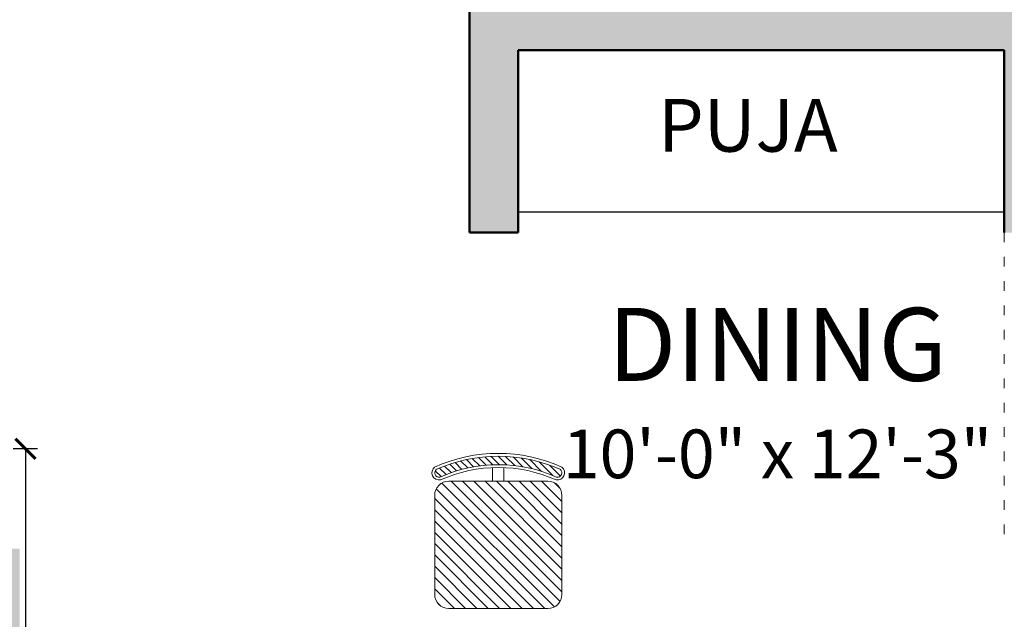
# Model space of a CAD drawing. Units: inches. Extents: x 375 to 1122, y 27 to 1069.
# Tile 66 of 155: x 667 to 788, y 326 to 400. Entities that reach past the tile are written whole.
import ezdxf

# ---------------------------------------------------------------- set-up
doc = ezdxf.new("R2010")
doc.units = ezdxf.units.IN
doc.linetypes.add('ACAD_ISO03W100', pattern=[30, 12, -18])
for name, color, linetype, lineweight in [('A-ANNO-DIMS', 2, 'Continuous', 18), ('A-AREA-IDEN', 7, 'Continuous', 18), ('A-COLS-PATT', 10, 'Continuous', 13), ('A-FLOR-MILL', 55, 'Continuous', 25), ('A-WALL-OVHD', 77, 'ACAD_ISO03W100', 18), ('A-WALL-PATT', 252, 'Continuous', 13), ('Furniture', 30, 'Continuous', 18), ('Walls', 250, 'Continuous', 50)]:
    doc.layers.add(name, color=color, linetype=linetype, lineweight=lineweight)
doc.styles.get("Standard").update_dxf_attribs({"font": 'arial.ttf'})
doc.dimstyles.new('ISO-25', dxfattribs={"dimtxt": 12, "dimasz": 2.5, "dimexe": 1.5, "dimexo": 1.5, "dimtad": 1, "dimdec": 1, "dimlunit": 3, "dimtxsty": 'Standard', "dimblk": 'ARCHTICK', "dimcen": 2.5, "dimadec": 0, "dimazin": 0, "dimtfac": 1, "dimtdec": 1, "dimtmove": 0, "dimatfit": 3, "dimfxl": 1.5, "dimfxlon": 1, "dimarcsym": 0})

# ---------------------------------------------------------------- blocks, each defined once
blk = doc.blocks.new('A$C403C54AD')
at = {"ltscale": 0.05}
for p, q in [((0.0699, 1.2072, -0.0006), (0.0361, 1.1733, -0.0006)), ((0.4273, 1.212, -0.0006), (0.0859, 0.8705, -0.0006)), ((0.3925, 1.212, -0.0006), (0.0859, 0.9053, -0.0006)), ((0.3576, 1.212, -0.0006), (0.0859, 0.9402, -0.0006)), ((0.3228, 1.212, -0.0006), (0.0859, 0.975, -0.0006)), ((0.288, 1.212, -0.0006), (0.0859, 1.0098, -0.0006)), ((0.2532, 1.212, -0.0006), (0.0859, 1.0447, -0.0006)), ((0.2183, 1.212, -0.0006), (0.0859, 1.0795, -0.0006)), ((0.1835, 1.212, -0.0006), (0.0859, 1.1143, -0.0006)), ((0.1487, 1.212, -0.0006), (0.0859, 1.1491, -0.0006)), ((0.1084, 1.2065, -0.0006), (0.0913, 1.1894, -0.0006)), ((0.4564, 1.2063, -0.0006), (0.0916, 0.8414, -0.0006)), ((0.4736, 1.1886, -0.0006), (0.1093, 0.8243, -0.0006)), ((0.068, 1.1835, -0.0006), (0.0259, 1.1414, -0.0006)), ((0.4785, 1.1587, -0.0006), (0.1391, 0.8193, -0.0006)), ((0.0556, 1.1493, -0.0006), (0.0189, 1.1126, -0.0006)), ((0.0472, 1.1192, -0.0006), (0.014, 1.086, -0.0006)), ((0.4785, 1.1239, -0.0006), (0.1739, 0.8193, -0.0006)), ((0.0378, 1.0663, -0.0006), (0.0092, 1.0377, -0.0006)), ((0.0415, 1.0917, -0.0006), (0.0109, 1.0612, -0.0006)), ((0.4785, 1.0891, -0.0006), (0.2088, 0.8193, -0.0006)), ((0.0357, 1.0424, -0.0006), (0.0087, 1.0154, -0.0006)), ((0.4785, 1.0542, -0.0006), (0.2436, 0.8193, -0.0006)), ((0.0349, 1.0198, -0.0006), (0.0092, 0.9941, -0.0006)), ((0.4785, 1.0194, -0.0006), (0.2784, 0.8193, -0.0006)), ((0.0352, 0.9984, -0.0006), (0.0106, 0.9737, -0.0006)), ((0.0365, 0.9779, -0.0006), (0.0128, 0.9542, -0.0006)), ((0.4785, 0.9846, -0.0006), (0.3133, 0.8193, -0.0006)), ((0.0386, 0.9582, -0.0006), (0.0157, 0.9353, -0.0006)), ((0.4785, 0.9497, -0.0006), (0.3481, 0.8193, -0.0006)), ((0.0415, 0.9394, -0.0006), (0.0192, 0.917, -0.0006)), ((0.0451, 0.9212, -0.0006), (0.0234, 0.8994, -0.0006)), ((0.4785, 0.9149, -0.0006), (0.3829, 0.8193, -0.0006)), ((0.0493, 0.9036, -0.0006), (0.0281, 0.8824, -0.0006)), ((0.0541, 0.8867, -0.0006), (0.0333, 0.8658, -0.0006)), ((0.0595, 0.8702, -0.0006), (0.039, 0.8498, -0.0006)), ((0.0653, 0.8543, -0.0006), (0.0452, 0.8342, -0.0006)), ((0.4785, 0.8801, -0.0006), (0.4177, 0.8193, -0.0006)), ((0.0717, 0.8389, -0.0006), (0.0537, 0.8209, -0.0006)), ((0.4692, 0.8359, -0.0006), (0.4619, 0.8287, -0.0006))]:
    blk.add_line(p, q, dxfattribs=at)
for p, q in [((0.1295, 1.212, -0.0006), (0.4349, 1.212, -0.0006)), ((0.0859, 0.8629, -0.0006), (0.0859, 1.1683, -0.0006)), ((0.4785, 1.1683, -0.0006), (0.4785, 0.8629, -0.0006)), ((0.0859, 1.0331, -0.0006), (0.0436, 1.0331, -0.0006)), ((0.0859, 0.9982, -0.0006), (0.0436, 0.9982, -0.0006)), ((0.304, 0.8193, -0.0006), (0.1295, 0.8193, -0.0006)), ((0.4349, 0.8193, -0.0006), (0.304, 0.8193, -0.0006))]:
    blk.add_line(p, q)
for centre, radius, start, end in [((0.0598, 1.1978, -0.0006), 0.0225, 350.3316, 141.1036), ((0.4774, 1.0156, -0.0006), 0.4774, 155.7176, 204.2824), ((0.4774, 1.0156, -0.0006), 0.4687, 155.7176, 204.2824), ((0.4774, 1.0156, -0.0006), 0.4425, 155.7176, 204.2824), ((0.4774, 1.0156, -0.0006), 0.4338, 155.7176, 204.2824), ((0.0598, 1.1978, -0.0006), 0.0138, 350.3316, 141.1036), ((0.1295, 1.1683, -0.0006), 0.0436, 90, 180), ((0.4349, 1.1683, -0.0006), 0.0436, 0, 90), ((0.1295, 0.8629, -0.0006), 0.0436, 180, 270), ((0.4349, 0.8629, -0.0006), 0.0436, 270, 0), ((0.0599, 0.8332, -0.0006), 0.0225, 218.3306, 10.2342), ((0.0599, 0.8332, -0.0006), 0.0138, 218.3306, 10.2342)]:
    blk.add_arc(centre, radius, start, end)
blk = doc.blocks.new('_ArchTick')
at = {"color": 0, "linetype": 'ByBlock', "const_width": 0.15}
blk.add_lwpolyline([(-0.5, -0.5), (0.5, 0.5)], dxfattribs=at)
blk = doc.blocks.new('*D59')
at = {"layer": 'A-ANNO-DIMS', "color": 0, "lineweight": -2, "transparency": 16777216}
for p, q in [((668.72, 346.85), (665.72, 346.85)), ((667.22, 346.85), (667.22, 232.35)), ((668.72, 232.35), (665.72, 232.35)), ((667.22, 232.35), (667.22, 27.5))]:
    blk.add_line(p, q, dxfattribs=at)
at = {"layer": 'Defpoints', "color": 0, "transparency": 16777216}
for p in [(684.39, 346.85), (667.22, 232.35), (684.39, 232.35)]:
    blk.add_point(p, dxfattribs=at)
at = {"layer": 'A-ANNO-DIMS', "color": 0, "lineweight": -2, "transparency": 16777216, "xscale": 2.5, "yscale": 2.5, "zscale": 2.5}
for p, rotation in [((667.22, 346.85), 90), ((667.22, 232.35), 270)]:
    blk.add_blockref('_ArchTick', p, dxfattribs=dict(at, rotation=rotation))
at = {"layer": 'A-ANNO-DIMS', "color": 0, "transparency": 16777216, "insert": (660.39, 128.67), "char_height": 12, "attachment_point": 5, "rotation": 90}
blk.add_mtext('DINING SET 9\'-6 1/2" TYP.', dxfattribs=at)
blk = doc.blocks.new('*D94')
at = {"layer": 'A-ANNO-DIMS', "color": 0, "lineweight": -2, "transparency": 16777216}
for p, q in [((734.01, 117.53), (734.01, 114.53)), ((773.01, 117.53), (773.01, 114.53)), ((734.01, 116.03), (773.01, 116.03))]:
    blk.add_line(p, q, dxfattribs=at)
at = {"layer": 'Defpoints', "color": 0, "transparency": 16777216}
for p in [(734.01, 667.53), (773.01, 667.53), (773.01, 116.03)]:
    blk.add_point(p, dxfattribs=at)
at = {"layer": 'A-ANNO-DIMS', "color": 0, "lineweight": -2, "transparency": 16777216, "xscale": 2.5, "yscale": 2.5, "zscale": 2.5, "rotation": 180}
blk.add_blockref('_ArchTick', (734.01, 116.03), dxfattribs=at)
at = {"layer": 'A-ANNO-DIMS', "color": 0, "lineweight": -2, "transparency": 16777216, "xscale": 2.5, "yscale": 2.5, "zscale": 2.5}
blk.add_blockref('_ArchTick', (773.01, 116.03), dxfattribs=at)
at = {"layer": 'A-ANNO-DIMS', "color": 0, "transparency": 16777216, "insert": (753.51, 122.78), "char_height": 12, "attachment_point": 5}
blk.add_mtext('3\'-3"', dxfattribs=at)

msp = doc.modelspace()

# ---------------------------------------------------------------- hatches: boundary and pattern name
at = {"layer": 'A-COLS-PATT'}
h = msp.add_hatch(color=256, dxfattribs=at)
h.dxf.hatch_style = 1
h.paths.add_polyline_path([(512.51, 982.53), (498.51, 982.53), (498.51, 973.53), (512.51, 973.53)])
h.paths.add_polyline_path([(666.51, 982.53), (652.51, 982.53), (652.51, 973.53), (666.51, 973.53)])
h.paths.add_polyline_path([(802.01, 982.53), (788.01, 982.53), (788.01, 973.53), (802.01, 973.53)])
h.paths.add_polyline_path([(932.01, 982.53), (918.01, 982.53), (918.01, 973.53), (932.01, 973.53)])
h.paths.add_polyline_path([(507.51, 841.53), (498.51, 841.53), (498.51, 827.53), (507.51, 827.53)])
h.paths.add_polyline_path([(666.51, 844.53), (652.51, 844.53), (652.51, 835.53), (666.51, 835.53)])
h.paths.add_polyline_path([(802.01, 814.53), (788.01, 814.53), (788.01, 805.53), (802.01, 805.53)])
h.paths.add_polyline_path([(932.01, 814.53), (918.01, 814.53), (918.01, 805.53), (932.01, 805.53)])
h.paths.add_polyline_path([(507.51, 719.53), (498.51, 719.53), (498.51, 705.53), (507.51, 705.53)])
h.paths.add_polyline_path([(731.01, 676.53), (722.01, 676.53), (722.01, 662.53), (731.01, 662.53)])
h.paths.add_polyline_path([(802.01, 676.53), (788.01, 676.53), (788.01, 667.53), (802.01, 667.53)])
h.paths.add_polyline_path([(932.01, 676.53), (918.01, 676.53), (918.01, 667.53), (932.01, 667.53)])
h.paths.add_polyline_path([(932.01, 583.53), (918.01, 583.53), (918.01, 574.53), (932.01, 574.53)])
h.paths.add_polyline_path([(868.01, 583.53), (854.01, 583.53), (854.01, 574.53), (868.01, 574.53)])
h.paths.add_polyline_path([(868.01, 502.53), (854.01, 502.53), (854.01, 493.53), (868.01, 493.53)])
h.paths.add_polyline_path([(932.01, 502.53), (918.01, 502.53), (918.01, 493.53), (932.01, 493.53)])
h.paths.add_polyline_path([(672.51, 592.03), (663.51, 592.03), (663.51, 578.03), (672.51, 578.03)])
h.paths.add_polyline_path([(512.51, 589.53), (498.51, 589.53), (498.51, 580.53), (512.51, 580.53)])
h.paths.add_polyline_path([(507.51, 464.53), (498.51, 464.53), (498.51, 450.53), (507.51, 450.53)])
h.paths.add_polyline_path([(731.01, 507.53), (722.01, 507.53), (722.01, 493.53), (731.01, 493.53)])
h.paths.add_polyline_path([(802.01, 502.53), (788.01, 502.53), (788.01, 493.53), (802.01, 493.53)])
h.paths.add_polyline_path([(507.51, 342.53), (498.51, 342.53), (498.51, 328.53), (507.51, 328.53)])
h.paths.add_polyline_path([(512.51, 196.53), (498.51, 196.53), (498.51, 187.53), (512.51, 187.53)])
h.paths.add_polyline_path([(666.51, 334.53), (652.51, 334.53), (652.51, 325.53), (666.51, 325.53)])
h.paths.add_polyline_path([(666.51, 196.53), (652.51, 196.53), (652.51, 187.53), (666.51, 187.53)])
h.paths.add_polyline_path([(805.01, 196.53), (791.01, 196.53), (791.01, 187.53), (805.01, 187.53)])
h.paths.add_polyline_path([(932.01, 196.53), (918.01, 196.53), (918.01, 187.53), (932.01, 187.53)])
h.paths.add_polyline_path([(932.01, 334.53), (918.01, 334.53), (918.01, 325.53), (932.01, 325.53)])
h.paths.add_polyline_path([(805.01, 334.53), (791.01, 334.53), (791.01, 325.53), (805.01, 325.53)])
at = {"layer": 'A-WALL-PATT'}
h = msp.add_hatch(color=256, dxfattribs=at)
h.dxf.hatch_style = 1
h.paths.add_polyline_path([(962.01, 388.53), (989.01, 388.53), (989.01, 394.53), (962.01, 394.53), (932.01, 394.53), (932.01, 397.53), (923.01, 397.53), (923.01, 394.53), (842.01, 394.53), (842.01, 334.53), (839.51, 334.53), (839.51, 328.53), (854.01, 328.53), (854.01, 334.53), (848.01, 334.53), (848.01, 388.53), (953.01, 388.53), (953.01, 356.08), (962.01, 356.08), (962.01, 358.55), (989.01, 358.55), (989.01, 364.55), (962.01, 364.55)])
h.paths.add_polyline_path([(989.01, 502.53), (932.01, 502.53), (932.01, 583.53), (932.01, 593.53), (923.01, 593.53), (923.01, 583.53), (854.01, 583.53), (854.01, 556.53), (863.01, 556.53), (863.01, 574.53), (923.01, 574.53), (923.01, 502.53), (863.01, 502.53), (863.01, 520.53), (854.01, 520.53), (854.01, 502.53), (773.01, 502.53), (773.01, 493.53), (788.01, 493.53), (788.01, 402.03), (722.01, 402.03), (722.01, 373.53), (728.01, 373.53), (728.01, 396.03), (788.01, 396.03), (788.01, 373.53), (794.01, 373.53), (794.01, 430.53), (814.01, 430.53), (814.01, 436.53), (794.01, 436.53), (794.01, 493.53), (923.01, 493.53), (923.01, 487.53), (932.01, 487.53), (932.01, 493.53), (983.01, 493.53), (983.01, 473.53), (989.01, 473.53)])
h.paths.add_polyline_path([(797.01, 325.53), (805.01, 325.53), (805.01, 328.53), (807.51, 328.53), (807.51, 334.53), (791.01, 334.53), (791.01, 226.53), (770.76, 226.53), (770.76, 217.53), (791.01, 217.53), (791.01, 187.53), (855.01, 187.53), (855.01, 196.53), (797.01, 196.53)])
h.paths.add_polyline_path([(989.01, 238.53), (962.01, 238.53), (962.01, 256.42), (953.01, 256.42), (953.01, 229.53), (980.01, 229.53), (980.01, 196.53), (915.01, 196.53), (915.01, 187.53), (989.01, 187.53)])
h.paths.add_polyline_path([(962.01, 334.53), (884.01, 334.53), (884.01, 328.53), (918.01, 328.53), (918.01, 325.53), (932.01, 325.53), (932.01, 328.53), (953.01, 328.53), (953.01, 304.42), (962.01, 304.42)])
h.paths.add_polyline_path([(606.51, 283.53), (609.51, 283.53), (609.51, 289.53), (600.51, 289.53), (600.51, 196.53), (578.51, 196.53), (578.51, 187.53), (606.51, 187.53), (606.51, 196.53)])
h.paths.add_polyline_path([(666.51, 292.53), (660.51, 292.53), (660.51, 289.53), (633.51, 289.53), (633.51, 283.53), (660.51, 283.53), (660.51, 196.53), (628.01, 196.53), (628.01, 187.53), (630.53, 187.53), (630.53, 160.53), (636.53, 160.53), (636.53, 187.53), (660.51, 187.53), (660.51, 160.53), (666.51, 160.53), (666.51, 217.53), (686.76, 217.53), (686.76, 226.53), (666.51, 226.53)])
h.paths.add_polyline_path([(480.51, 256.42), (471.51, 256.42), (471.51, 238.53), (444.51, 238.53), (444.51, 187.53), (518.51, 187.53), (518.51, 196.53), (453.51, 196.53), (453.51, 229.53), (480.51, 229.53)])
h.paths.add_polyline_path([(480.51, 328.53), (652.51, 328.53), (652.51, 325.53), (660.51, 325.53), (660.51, 322.53), (666.51, 322.53), (666.51, 334.53), (507.51, 334.53), (507.51, 360.53), (498.51, 360.53), (498.51, 334.53), (471.51, 334.53), (471.51, 304.42), (480.51, 304.42)])
h.paths.add_polyline_path([(507.51, 484.53), (498.51, 484.53), (498.51, 444.53), (507.51, 444.53), (507.51, 454.53), (621.51, 454.53), (621.51, 460.53), (507.51, 460.53)])
h.paths.add_polyline_path([(672.51, 604.53), (683.26, 604.53), (683.26, 613.53), (669.51, 613.53), (669.51, 649.53), (663.51, 649.53), (663.51, 589.53), (507.51, 589.53), (507.51, 613.53), (498.51, 613.53), (498.51, 556.53), (507.51, 556.53), (507.51, 580.53), (663.51, 580.53), (663.51, 520.53), (669.51, 520.53), (669.51, 556.53), (683.26, 556.53), (683.26, 565.53), (672.51, 565.53)])
h.paths.add_polyline_path([(731.01, 667.53), (734.01, 667.53), (734.01, 676.53), (728.01, 676.53), (728.01, 715.53), (657.51, 715.53), (657.51, 709.53), (663.51, 709.53), (663.51, 673.53), (669.51, 673.53), (669.51, 709.53), (722.01, 709.53), (722.01, 613.53), (704.76, 613.53), (704.76, 604.53), (722.01, 604.53), (722.01, 565.53), (704.76, 565.53), (704.76, 556.53), (722.01, 556.53), (722.01, 502.53), (722.01, 460.53), (669.51, 460.53), (669.51, 496.53), (663.51, 496.53), (663.51, 460.53), (657.51, 460.53), (657.51, 454.53), (728.01, 454.53), (728.01, 493.53), (734.01, 493.53), (734.01, 502.53), (731.01, 502.53)])
h.paths.add_polyline_path([(986.01, 718.53), (959.01, 718.53), (959.01, 727.53), (950.01, 727.53), (950.01, 709.53), (977.01, 709.53), (977.01, 676.53), (794.01, 676.53), (794.01, 805.53), (802.01, 805.53), (802.01, 808.53), (804.51, 808.53), (804.51, 814.53), (788.01, 814.53), (788.01, 774.03), (728.01, 774.03), (728.01, 796.53), (722.01, 796.53), (722.01, 768.03), (788.01, 768.03), (788.01, 676.53), (773.01, 676.53), (773.01, 667.53), (923.01, 667.53), (923.01, 657.53), (932.01, 657.53), (932.01, 667.53), (986.01, 667.53)])
h.paths.add_polyline_path([(621.51, 715.53), (507.51, 715.53), (507.51, 733.53), (498.51, 733.53), (498.51, 715.53), (498.51, 685.53), (507.51, 685.53), (507.51, 709.53), (621.51, 709.53)])
h.paths.add_polyline_path([(666.51, 847.03), (660.51, 847.03), (660.51, 844.53), (652.51, 844.53), (652.51, 841.53), (480.51, 841.53), (480.51, 859.53), (471.51, 859.53), (471.51, 835.53), (498.51, 835.53), (498.51, 817.53), (507.51, 817.53), (507.51, 835.53), (666.51, 835.53)])
h.paths.add_polyline_path([(480.51, 940.53), (453.51, 940.53), (453.51, 973.53), (518.51, 973.53), (518.51, 982.53), (444.51, 982.53), (444.51, 931.53), (471.51, 931.53), (471.51, 907.53), (480.51, 907.53)])
h.paths.add_polyline_path([(606.51, 982.53), (578.51, 982.53), (578.51, 973.53), (600.51, 973.53), (600.51, 880.53), (609.51, 880.53), (609.51, 886.53), (606.51, 886.53)])
h.paths.add_polyline_path([(666.51, 943.53), (686.76, 943.53), (686.76, 952.53), (666.51, 952.53), (666.51, 1009.53), (660.51, 1009.53), (660.51, 982.53), (636.53, 982.53), (636.53, 1009.53), (630.53, 1009.53), (630.53, 982.53), (628.01, 982.53), (628.01, 973.53), (660.51, 973.53), (660.51, 886.53), (633.51, 886.53), (633.51, 880.53), (660.51, 880.53), (660.51, 877.03), (666.51, 877.03)])
h.paths.add_polyline_path([(986.01, 874.53), (932.01, 874.53), (932.01, 877.53), (923.01, 877.53), (923.01, 874.53), (788.01, 874.53), (788.01, 868.53), (788.01, 844.53), (794.01, 844.53), (794.01, 868.53), (839.01, 868.53), (839.01, 814.53), (836.51, 814.53), (836.51, 808.53), (851.01, 808.53), (851.01, 814.53), (845.01, 814.53), (845.01, 868.53), (986.01, 868.53)])
h.paths.add_polyline_path([(959.01, 838.55), (986.01, 838.55), (986.01, 844.55), (959.01, 844.55), (959.01, 847.03), (950.01, 847.03), (950.01, 814.53), (881.01, 814.53), (881.01, 808.53), (918.01, 808.53), (918.01, 805.53), (932.01, 805.53), (932.01, 808.53), (950.01, 808.53), (950.01, 793.53), (959.01, 793.53)])
h.paths.add_polyline_path([(986.01, 982.53), (899.01, 982.53), (899.01, 973.53), (923.01, 973.53), (923.01, 967.53), (932.01, 967.53), (932.01, 973.53), (980.01, 973.53), (980.01, 953.53), (986.01, 953.53)])
h.paths.add_polyline_path([(851.01, 982.53), (788.01, 982.53), (788.01, 952.53), (770.76, 952.53), (770.76, 943.53), (788.01, 943.53), (788.01, 910.53), (814.01, 910.53), (814.01, 916.53), (794.01, 916.53), (794.01, 973.53), (851.01, 973.53)])

# ---------------------------------------------------------------- linework, layer by layer
at = {"layer": 'A-FLOR-MILL'}
msp.add_line((788.01, 376.03), (728.01, 376.03), dxfattribs=at)
at = {"layer": 'A-WALL-OVHD', "ltscale": 0.1}
msp.add_line((788.01, 373.53), (788.01, 334.53), dxfattribs=at)
at = {"layer": 'Walls'}
for p, q in [((722.01, 373.53), (722.01, 402.03)), ((728.01, 373.53), (728.01, 396.03)), ((788.01, 396.03), (728.01, 396.03)), ((788.01, 373.53), (788.01, 396.03)), ((722.01, 373.53), (728.01, 373.53))]:
    msp.add_line(p, q, dxfattribs=at)

# ---------------------------------------------------------------- block references
at = {"layer": 'Furniture', "xscale": 39.9918517141215, "yscale": 39.9918517141215, "zscale": 39.9918517141215, "rotation": 270}
msp.add_blockref('A$C403C54AD', (684.95, 346.29, 0.02), dxfattribs=at)

# ---------------------------------------------------------------- texts
at = {"layer": 'A-AREA-IDEN', "attachment_point": 1}
for s, width, insert, char_height in [('\\pxqc;{\\fArial|b1|i0|c0|p34;PUJA}', 42.2291, (735.26, 390), 6.5), ('\\pxqc;{\\fArial|b1|i0|c0|p34;\\H0.75x;DINING\\H1.33333x;\\P\\fArial|b0|i0|c0|p34;\\H0.5x;10\'-0" x 12\'-3"}', 66.1169, (726.96, 364.23), 12)]:
    msp.add_mtext_dynamic_manual_height_columns(s, width=width, gutter_width=12.5, heights=[0], dxfattribs=dict(at, insert=insert, char_height=char_height))

# ---------------------------------------------------------------- dimensions: what is measured, and where the dimension line sits
at = {"layer": 'A-ANNO-DIMS'}
dim = msp.add_linear_dim(base=(773.01, 116.03), p1=(734.01, 667.53), p2=(773.01, 667.53), dimstyle='ISO-25', override={"dimdec": 1, "dimlfac": 1, "dimrnd": 0, "dimzin": 1, "dimdsep": 46, "dimlunit": 4, "dimfrac": 2}, dxfattribs=at)
dim.commit()
dim.dimension.update_dxf_attribs({"geometry": '*D94', "text_midpoint": (753.51, 122.78)})
dim = msp.add_linear_dim(base=(667.22, 232.35), p1=(684.39, 346.85), p2=(684.39, 232.35), angle=270, text='DINING SET <> TYP.', dimstyle='ISO-25', override={"dimdec": 1, "dimlfac": 1, "dimrnd": 0, "dimzin": 1, "dimdsep": 46, "dimlunit": 4, "dimfrac": 2}, dxfattribs=at)
dim.commit()
dim.dimension.update_dxf_attribs({"geometry": '*D59', "text_midpoint": (660.39, 128.67)})

doc.saveas('drawing.dxf')
